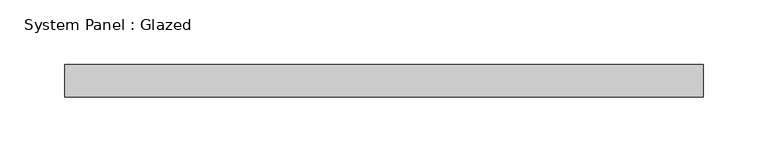
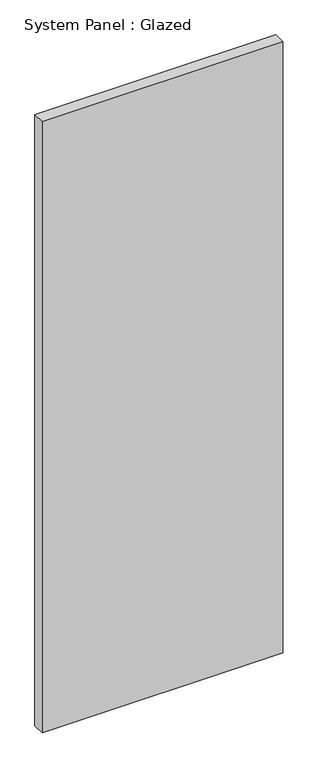
"""IFC4 building model written with IfcOpenShell, lengths in millimetres: plate geometry, System Panel : Glazed."""

from ifc_helpers import new_model, si_unit, origin, origin_with_axes, place, context, project, spatial, polyline, outline, extrude, source, transform, mapped, element, save


def system_panel_glazed_eaaab531(model_context):
    return source(origin(), model_context, "Body", "SweptSolid", [
        extrude(outline(polyline([(247.65, 19.05), (-247.65, 19.05), (-247.65, 44.45), (247.65, 44.45), (247.65, 19.05)])), origin_with_axes(), (0.0, 0.0, 1.0), 1329.6512079),
    ])


if __name__ == "__main__":
    model = new_model("IFC4")
    model_context = context("Model", 3, world=origin())
    ifc_project = project(units=[si_unit("LENGTHUNIT", "METRE", prefix="MILLI")], contexts=[model_context])
    site = spatial("IfcSite", under=ifc_project)
    building = spatial("IfcBuilding", under=site)
    placement = place(None, origin())
    system_panel_glazed_shape = system_panel_glazed_eaaab531(model_context)
    element("IfcPlate", 1, ObjectType="System Panel : Glazed", at=placement, inside=building, context=model_context, shape_type="MappedRepresentation", body=[
        mapped(system_panel_glazed_shape, transform((0.0, 0.0, 0.0), x_axis=(1.0, 0.0, 0.0), y_axis=(0.0, 1.0, 0.0), z_axis=(0.0, 0.0, 1.0))),
    ])
    save(model, "model.ifc")

# Revit data of these elements
# Type "System Panel : Glazed"
#   Construction Type Id = "GSP4R"
#   Analytic Construction = "1/8 in Pilkington single glazing"
#   Visual Light Transmittance = 0.9
#   Solar Heat Gain Coefficient = 0.86
#   Heat Transfer Coefficient (U) = 1.18115 BTU/(h·ft²·°F)
#   Define Thermal Properties by = 1
# Element 1 (IfcPlate, "System Panel : Glazed")
#   Materials on its faces: "Glass"
# Materials
#   "Glass": class "Glass", colour RGB 0 128 192, transparency 0.75, Description = "Soda Lime Glass", Cost = 0
